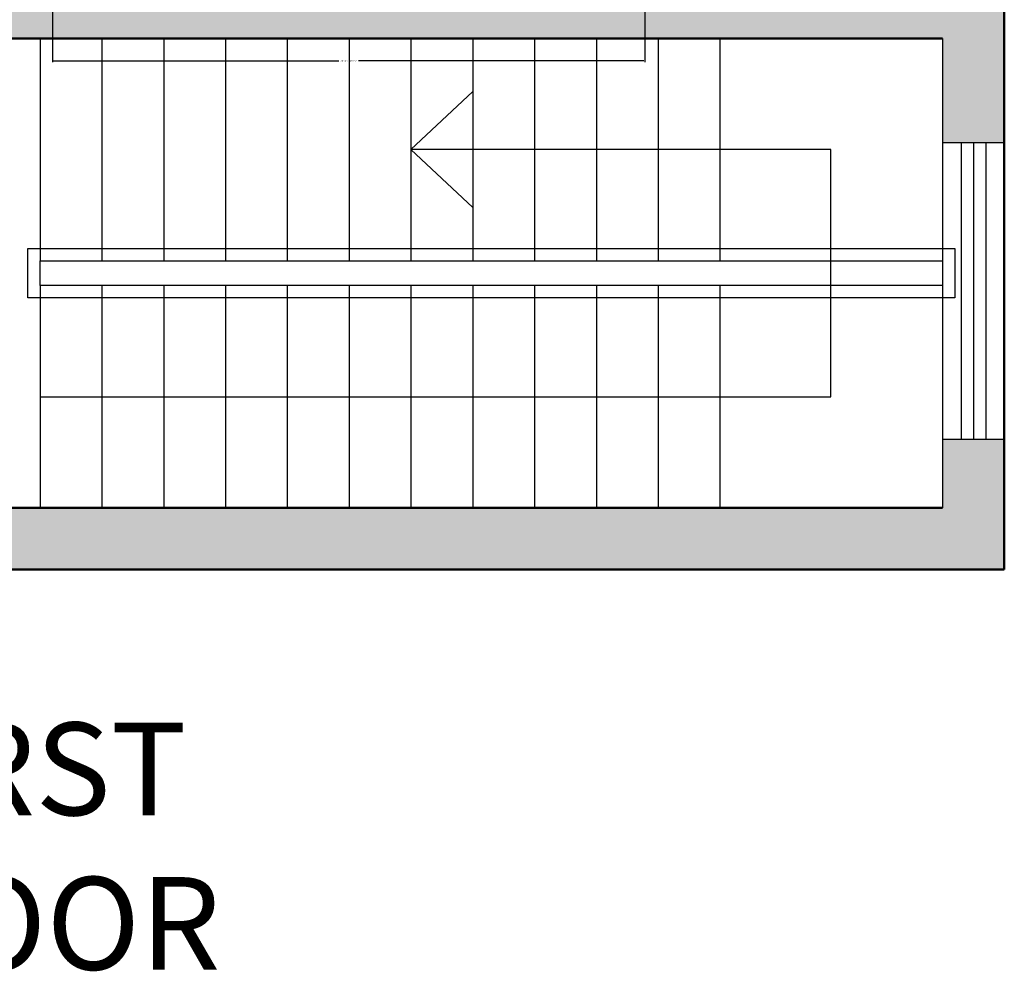
# Model space of a CAD drawing. Units: inches. Extents: x 1771 to 3025, y 319 to 889.
# Tile 14 of 35: x 2402 to 2561, y 319 to 473. Entities that reach past the tile are written whole.
import ezdxf

# ---------------------------------------------------------------- set-up
doc = ezdxf.new("R2010")
doc.units = ezdxf.units.IN
doc.header["$MEASUREMENT"] = 0
for name, color, linetype, lineweight in [('A-ANNO-DIMS', 2, 'Continuous', 18), ('A-AREA-IDEN', 241, 'Continuous', 25), ('A-FLOR-STRS', 7, 'Continuous', 25), ('A-GLAZ', 40, 'Continuous', 25), ('A-WALL', 7, 'Continuous', 50), ('A-WALL-PATT', 254, 'Continuous', 13)]:
    doc.layers.add(name, color=color, linetype=linetype, lineweight=lineweight)
doc.styles.get("Standard").update_dxf_attribs({"font": 'arial.ttf'})
doc.dimstyles.get("Standard").update_dxf_attribs({"dimtxt": 0.18, "dimasz": 0.18, "dimexe": 0.18, "dimexo": 0.0625, "dimgap": 0.09, "dimtad": 0, "dimtih": 1, "dimtoh": 1, "dimdec": 4, "dimzin": 0, "dimdsep": 46, "dimtxsty": 'Standard', "dimcen": 0.09, "dimadec": 0, "dimazin": 0, "dimtfac": 1, "dimtdec": 4, "dimtofl": 0, "dimtmove": 0, "dimatfit": 3, "dimfxl": 1, "dimtolj": 1, "dimtzin": 0, "dimarcsym": 0})

# ---------------------------------------------------------------- blocks, each defined once
blk = doc.blocks.new('WIN-48')
for p, q in [((0, 0), (0, 10)), ((48, 0), (48, 10)), ((0, 7), (48, 7)), ((0, 5), (48, 5)), ((0, 3), (48, 3))]:
    blk.add_line(p, q)
blk = doc.blocks.new('*D42')
at = {"layer": 'A-ANNO-DIMS', "color": 0, "lineweight": -2, "transparency": 16777216}
for p, q in [((2407.16, 480.28), (2407.16, 465.79)), ((2503, 480.28), (2503, 465.79)), ((2407.34, 465.97), (2453.48, 465.97)), ((2502.82, 465.97), (2456.68, 465.97))]:
    blk.add_line(p, q, dxfattribs=at)
at = {"layer": 'A-ANNO-DIMS', "color": 0, "transparency": 16777216}
for points in [[(2407.34, 466), (2407.34, 465.94), (2407.16, 465.97)], [(2502.82, 466), (2502.82, 465.94), (2503, 465.97)]]:
    blk.add_solid(points, dxfattribs=at)
at = {"layer": 'Defpoints', "color": 0, "transparency": 16777216}
for p in [(2407.16, 480.34), (2503, 480.34), (2503, 465.97)]:
    blk.add_point(p, dxfattribs=at)
at = {"layer": 'A-ANNO-DIMS', "color": 0, "transparency": 16777216, "insert": (2455.08, 465.97), "char_height": 0.18, "attachment_point": 5}
blk.add_mtext('\\A1;LOUNGE CHAIRS 96 TYP.', dxfattribs=at)

msp = doc.modelspace()

# ---------------------------------------------------------------- hatches: boundary and pattern name
at = {"layer": 'A-WALL-PATT'}
h = msp.add_hatch(color=256, dxfattribs=at)
h.dxf.hatch_style = 1
h.paths.add_polyline_path([(2407.16, 878.63), (2429.21, 878.63), (2429.21, 888.63), (2379.16, 888.63), (2379.16, 878.63), (2402.16, 878.63), (2402.16, 830.63), (2407.16, 830.63)])
h.paths.add_polyline_path([(2520.11, 888.63), (2477.21, 888.63), (2477.21, 878.63), (2498.16, 878.63), (2498.16, 794.63), (2402.16, 794.63), (2402.16, 758.63), (2402.16, 664.63), (2407.16, 664.63), (2407.16, 712), (2407.16, 789.63), (2515.16, 789.63), (2515.16, 794.63), (2503.16, 794.63), (2503.16, 878.63), (2520.11, 878.63)])
h.paths.add_polyline_path([(2561.16, 888.63), (2538.11, 888.63), (2538.11, 878.63), (2551.16, 878.63), (2551.16, 789.63), (2551.16, 768.61), (2561.16, 768.61)])
h.paths.add_polyline_path([(2561.16, 720.61), (2551.16, 720.61), (2551.16, 669.63), (2443.16, 669.63), (2443.16, 664.63), (2462.16, 664.63), (2462.16, 652.63), (2467.16, 652.63), (2467.16, 664.63), (2551.16, 664.63), (2551.16, 649.17), (2561.16, 649.17)])
h.paths.add_polyline_path([(2561.16, 631.17), (2551.16, 631.17), (2551.16, 616.63), (2462.16, 616.63), (2443.16, 616.63), (2443.16, 611.63), (2551.16, 611.63), (2551.16, 581.11), (2561.16, 581.11)])
h.paths.add_polyline_path([(2561.16, 533.11), (2551.16, 533.11), (2551.16, 479.63), (2407.16, 479.63), (2407.16, 616.63), (2397.16, 616.63), (2397.16, 543.63), (2306.16, 543.63), (2306.16, 533.63), (2397.16, 533.63), (2397.16, 469.63), (2551.16, 469.63), (2551.16, 452.76), (2561.16, 452.76)])
h.paths.add_polyline_path([(2561.16, 404.76), (2551.16, 404.76), (2551.16, 393.63), (2397.16, 393.63), (2397.16, 383.63), (2561.16, 383.63)])
h.paths.add_polyline_path([(2270.16, 642.58), (2260.16, 642.58), (2260.16, 533.63), (2270.16, 533.63)])
h.paths.add_polyline_path([(2270.16, 753.63), (2366.16, 753.63), (2366.16, 758.63), (2270.16, 758.63), (2270.16, 842.59, -0.008336), (2268.86, 842.63), (2260.16, 842.63), (2260.16, 690.58), (2270.16, 690.58)])
h.paths.add_polyline_path([(2331.16, 888.63), (2260.16, 888.63), (2260.16, 878.63), (2331.16, 878.63)])

# ---------------------------------------------------------------- linework, layer by layer
at = {"layer": 'A-FLOR-STRS'}
for p, q in [((2405.16, 469.63), (2405.16, 433.63)), ((2415.16, 469.63), (2415.16, 433.63)), ((2425.16, 469.63), (2425.16, 433.63)), ((2435.16, 469.63), (2435.16, 433.63)), ((2445.16, 469.63), (2445.16, 433.63)), ((2455.16, 469.63), (2455.16, 433.63)), ((2465.16, 469.63), (2465.16, 433.63)), ((2475.16, 469.63), (2475.16, 433.63)), ((2485.16, 469.63), (2485.16, 433.63)), ((2495.16, 469.63), (2495.16, 433.63)), ((2505.16, 469.63), (2505.16, 433.63)), ((2515.16, 469.63), (2515.16, 433.63)), ((2551.16, 469.63), (2551.16, 393.63)), ((2405.16, 429.63), (2405.16, 393.63)), ((2415.16, 429.63), (2415.16, 393.63)), ((2425.16, 429.63), (2425.16, 393.63)), ((2435.16, 429.63), (2435.16, 393.63)), ((2445.16, 429.63), (2445.16, 393.63)), ((2455.16, 429.63), (2455.16, 393.63)), ((2465.16, 429.63), (2465.16, 393.63)), ((2475.16, 429.63), (2475.16, 393.63)), ((2485.16, 429.63), (2485.16, 393.63)), ((2495.16, 429.63), (2495.16, 393.63)), ((2505.16, 429.63), (2505.16, 393.63)), ((2515.16, 429.63), (2515.16, 393.63))]:
    msp.add_line(p, q, dxfattribs=at)
for points in [[(2465.16, 451.63), (2475.16, 461.01)], [(2405.16, 411.63), (2533.08, 411.63), (2533.08, 451.63), (2465.16, 451.63)], [(2465.16, 451.63), (2475.16, 442.26)]]:
    msp.add_lwpolyline(points, dxfattribs=at)
for points in [[(2403.16, 435.63), (2553.14, 435.63), (2553.14, 427.63), (2403.16, 427.63)], [(2405.16, 433.63), (2551.14, 433.63), (2551.14, 429.63), (2405.16, 429.63)]]:
    msp.add_lwpolyline(points, close=True, dxfattribs=at)
at = {"layer": 'A-WALL'}
for p, q in [((2561.16, 383.63), (2561.16, 888.43)), ((2397.16, 469.63), (2551.16, 469.63)), ((2397.16, 393.63), (2551.16, 393.63)), ((2397.16, 383.63), (2561.16, 383.63))]:
    msp.add_line(p, q, dxfattribs=at)

# ---------------------------------------------------------------- block references
at = {"layer": 'A-GLAZ', "rotation": 270.0000000000006}
msp.add_blockref('WIN-48', (2551.16, 452.76), dxfattribs=at)

# ---------------------------------------------------------------- texts
at = {"layer": 'A-AREA-IDEN', "insert": (2358.75, 358.88), "char_height": 15, "attachment_point": 1}
msp.add_mtext_dynamic_manual_height_columns('\\pxqc;FIRST FLOOR ', width=85.4611, gutter_width=1, heights=[0], dxfattribs=at)

# ---------------------------------------------------------------- dimensions: what is measured, and where the dimension line sits
at = {"layer": 'A-ANNO-DIMS'}
dim = msp.add_linear_dim(base=(2503, 465.97), p1=(2407.16, 480.34), p2=(2503, 480.34), text='LOUNGE CHAIRS <> TYP.', dimstyle='Standard', override={"dimdec": 0, "dimrnd": 0, "dimzin": 0, "dimlunit": 2}, dxfattribs=at)
dim.commit()
dim.dimension.update_dxf_attribs({"geometry": '*D42', "text_midpoint": (2455.08, 465.97)})

doc.saveas('drawing.dxf')
